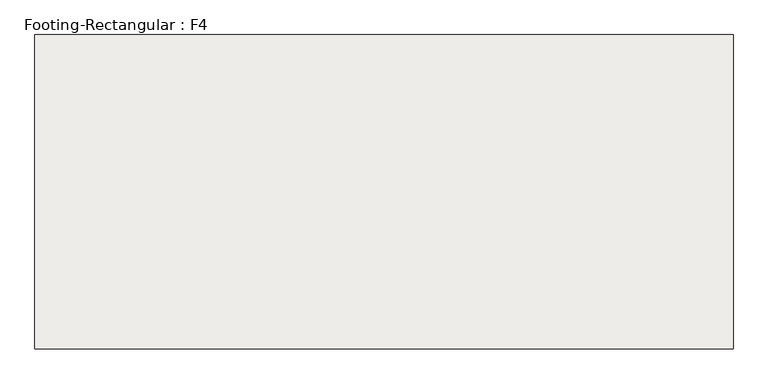
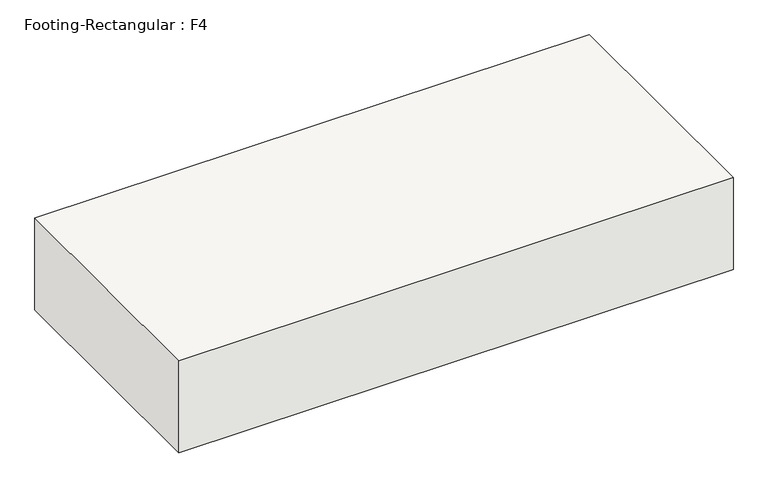
"""IFC4 building model written with IfcOpenShell, lengths in millimetres: slab geometry, Footing-Rectangular : F4."""

from ifc_helpers import new_model, si_unit, frame, origin, place, context, project, spatial, polyline, outline, extrude, source, transform, mapped, element, save


def footing_rectangular_f4_618a482d(model_context):
    return source(origin(), model_context, "Body", "SweptSolid", [
        extrude(outline(polyline([(1524.0, 685.8), (1524.0, -685.8), (-1524.0, -685.8), (-1524.0, 685.8), (1524.0, 685.8)])), frame((0.0, 0.0, -533.4), z_axis=(0.0, 0.0, 1.0), x_axis=(1.0, 0.0, 0.0)), (0.0, 0.0, 1.0), 533.4),
    ])


if __name__ == "__main__":
    model = new_model("IFC4")
    model_context = context("Model", 3, world=origin())
    ifc_project = project(units=[si_unit("LENGTHUNIT", "METRE", prefix="MILLI")], contexts=[model_context])
    site = spatial("IfcSite", under=ifc_project)
    building = spatial("IfcBuilding", under=site)
    placement = place(None, origin())
    footing_rectangular_f4_shape = footing_rectangular_f4_618a482d(model_context)
    element("IfcSlab", 1, ObjectType="Footing-Rectangular : F4", at=placement, inside=building, context=model_context, shape_type="MappedRepresentation", body=[
        mapped(footing_rectangular_f4_shape, transform((0.0, 0.0, 0.0), x_axis=(1.0, 0.0, 0.0), y_axis=(0.0, 1.0, 0.0), z_axis=(0.0, 0.0, 1.0))),
    ])
    save(model, "model.ifc")

# Revit data of these elements
# Type "Footing-Rectangular : F4"
#   Width = 3048 mm
#   Length = 1371.6 mm
#   Foundation Thickness = 533.4 mm
#   Structural Material [instance default] = Concrete - Cast-in-Place Concrete
#   Assembly Code = ""
# Element 1 (IfcSlab, "Footing-Rectangular : F4")
#   Materials on its faces: "Concrete - Cast-in-Place Concrete"
# Materials
#   "Concrete - Cast-in-Place Concrete": class "Concrete", colour RGB 192 192 192, transparency 0, Cost = 0
